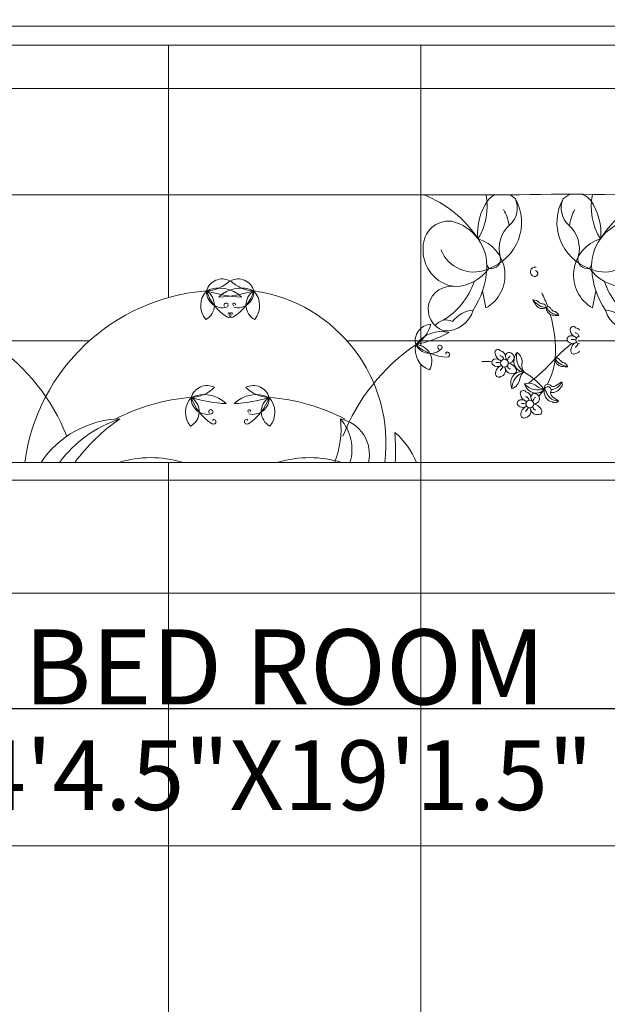
# Model space of a CAD drawing. Units: inches. Extents: x 351 to 1738, y -265 to 286.
# Tile 34 of 38: x 1448 to 1506, y 20 to 118. Entities that reach past the tile are written whole.
import ezdxf

# ---------------------------------------------------------------- set-up
doc = ezdxf.new("R2010")
doc.units = ezdxf.units.IN
doc.header["$MEASUREMENT"] = 0
for name, color, linetype, lineweight in [('A-ANNO-DIMS', 2, 'Continuous', 18), ('A-AREA-IDEN', 7, 'Continuous', 18), ('A-FLOR-PATT', 9, 'Continuous', 9), ('A-FURN', 18, 'Continuous', 13)]:
    doc.layers.add(name, color=color, linetype=linetype, lineweight=lineweight)
doc.styles.add('Annotative', font='arial.ttf')
doc.styles.get("Standard").update_dxf_attribs({"font": 'arial.ttf'})
doc.dimstyles.get("Standard").update_dxf_attribs({"dimtxt": 8, "dimasz": 5, "dimexe": 0.18, "dimexo": 0.0625, "dimgap": 0.09, "dimtad": 1, "dimtoh": 1, "dimzin": 0, "dimdsep": 46, "dimlunit": 4, "dimtxsty": 'Standard', "dimcen": 0, "dimclre": 256, "dimadec": 0, "dimazin": 0, "dimtfac": 1, "dimtofl": 0, "dimtmove": 0, "dimatfit": 3, "dimfxl": 1, "dimtolj": 1, "dimtzin": 0, "dimlwe": -1, "dimarcsym": 0})

# ---------------------------------------------------------------- blocks, each defined once
blk = doc.blocks.new('BED-DOUBLE-W-NIGHTSTANDS')
for p, q in [((121.406, 44.947), (28.441, 44.947)), ((121.549, 43.065), (28.441, 43.065)), ((106.084, 28.242), (44.816, 28.242)), ((102.765, 17.047), (102.431, 18.753)), ((113.311, 17.047), (113.645, 18.753))]:
    blk.add_line(p, q)
for points in [[(121.562, 54.359), (129.93, 54.359), (129.93, 0), (19.917, 0), (19.917, 54.359), (28.453, 54.359)], [(28.449, 52.61), (21.666, 52.61), (21.666, 1.749), (128.181, 1.749), (128.181, 52.61), (121.53, 52.61)]]:
    blk.add_lwpolyline(points)
for centre in [(104.593, 11.579), (107.107, 7.529)]:
    blk.add_circle(centre, 0.384)
for centre, radius, start, end in [((110.705, -118.523), 146.838, 85.24024, 91.80351), ((111.698, 26.573), 1.817, 106.63434, 135.54831), ((111.698, 26.573), 1.817, 37.67503, 72.58143), ((119.442, 27.126), 6.252, 169.24899, 211.17822), ((92.445, 17.616), 11.421, 33.66712, 68.50587), ((107.751, 24.412), 5.82, 145.78505, 184.73037), ((96.634, 27.126), 6.252, 328.82178, 10.28665), ((104.377, 26.573), 1.817, 113.28564, 142.32497), ((101.476, 25.502), 4.809, 289.28218, 29.1751), ((104.377, 26.573), 1.817, 44.45169, 66.71436), ((103.609, 26.933), 2.258, 311.56531, 23.83541), ((114.6, 25.502), 4.809, 150.8249, 250.71782), ((112.466, 26.933), 2.258, 156.16459, 228.43469), ((108.324, 24.412), 5.82, 355.26963, 34.21495), ((123.631, 17.616), 11.421, 113.64533, 146.33288), ((100.75, 24.631), 4.338, 7.43599, 29.91487), ((115.326, 24.631), 4.338, 150.08513, 172.56401), ((99.098, 23.1), 2.548, 84.48557, 181.05378), ((98.316, 21.215), 4.539, 355.29334, 76.921), ((117.76, 21.215), 4.539, 103.079, 184.70666), ((107.16, 22.929), 3.094, 131.56531, 195.14713), ((108.916, 22.929), 3.094, 344.85287, 48.43469), ((100.894, 20.299), 3.752, 299.90854, 73.1337), ((115.181, 20.299), 3.752, 106.8663, 240.09146), ((100.143, 22.735), 3.606, 174.94485, 262.88575), ((101.56, 24.102), 3.502, 201.58187, 291.42215), ((114.516, 24.102), 3.502, 248.57785, 338.41813), ((103.27, 21.876), 0.937, 257.30406, 15.14713), ((112.806, 21.876), 0.937, 164.85287, 282.69594), ((99.516, 23.537), 4.383, 272.3591, 324.04014), ((94.756, 21.336), 8.098, 326.28828, 356.5076), ((107.751, 24.412), 5.82, 212.70113, 216.34448), ((107.638, 20.635), 0.473, 79.58644, 259.56155), ((107.605, 20.456), 0.291, 259.56155, 77.29493), ((108.324, 24.412), 5.82, 323.65552, 327.29887), ((116.56, 23.537), 4.383, 215.95986, 267.6409), ((121.319, 21.336), 8.098, 183.4924, 213.71172), ((76.659, 18.283), 1.634, 63.02737, 163.80375), ((75.004, 22.103), 3.366, 271.45846, 315.37266), ((78.218, 18.283), 1.634, 16.19625, 116.97263), ((79.873, 22.103), 3.366, 224.62734, 268.54154), ((94.823, 21.91), 7.124, 301.26137, 341.7045), ((121.253, 21.91), 7.124, 198.2955, 238.73863), ((76.623, -0.907), 19.706, 94.46233, 172.25504), ((76.708, 17.271), 2.185, 137.78732, 219.11446), ((74.227, 17.338), 1.646, 298.5391, 58.36268), ((76.701, 18.676), 1.612, 177.75849, 283.85198), ((76.373, 15.9), 3.115, 45.54113, 114.31008), ((79.214, 31.893), 13.785, 252.59304, 267.25817), ((79.804, 20.354), 4.984, 198.91595, 238.01098), ((78.505, 15.9), 3.115, 65.68992, 134.45887), ((75.663, 31.893), 13.785, 272.74183, 287.40696), ((75.073, 20.354), 4.984, 301.98902, 341.08405), ((78.176, 18.676), 1.612, 256.14802, 2.24151), ((80.65, 17.338), 1.646, 121.63732, 241.4609), ((78.169, 17.271), 2.185, 320.88554, 42.21268), ((77.617, 3.643), 15.251, 352.86355, 81.81966), ((99.313, 16.925), 2.265, 80.26398, 250.86884), ((97.145, 12.86), 12.498, 20.10592, 26.9968), ((107.447, 17.052), 0.792, 39.50559, 92.64212), ((109.278, 19.327), 2.385, 218.43876, 238.83597), ((111.218, 19.743), 4.256, 206.50636, 215.31021), ((109.029, 19.778), 2.424, 246.39009, 254.48709), ((77.036, 17.318), 0.213, 283.85198, 219.92454), ((77.821, 17.4), 0.128, 320.19092, 256.02088), ((98.77, 17.606), 2.828, 265.96902, 344.3045), ((101.816, 13.847), 3.012, 96.1662, 141.58255), ((108.328, 17.714), 0.724, 216.52319, 302.46683), ((108.698, 18.368), 1.265, 238.83597, 270.81412), ((108.411, 17.136), 0.307, 353.94573, 95.62162), ((109.439, 17.049), 0.724, 175.71315, 261.65678), ((108.889, 16.849), 0.307, 22.55835, 124.23425), ((109.84, 17.685), 1.265, 207.36586, 239.34401), ((110.926, 18.642), 2.424, 223.69288, 231.78988), ((110.411, 18.648), 2.385, 239.34401, 259.74122), ((109.271, 15.96), 0.792, 25.53786, 78.67439), ((117.306, 17.606), 2.828, 195.6955, 274.03098), ((114.26, 13.847), 3.012, 38.41745, 83.8338), ((77.294, 16.335), 0.245, 238.01098, 71.55918), ((77.334, 16.455), 0.119, 71.55918, 188.01668), ((77.583, 16.335), 0.245, 108.44082, 301.98902), ((77.543, 16.455), 0.119, 351.98332, 108.44082), ((98.847, 14.471), 1.388, 63.97555, 143.26805), ((97.145, 12.86), 12.498, 356.17232, 16.41582), ((109.862, 20.555), 4.256, 262.86976, 271.67361), ((97.395, 13.794), 1.634, 92.95159, 193.72796), ((94.055, 16.28), 3.366, 301.38267, 345.29688), ((98.336, 11.586), 3.115, 75.46535, 144.23429), ((111.397, 14.916), 0.297, 35.0752, 194.76444), ((112.026, 14.961), 0.924, 187.49685, 251.27373), ((111.511, 14.458), 0.641, 37.3642, 78.43627), ((92.82, 26.864), 13.785, 282.51726, 297.18239), ((111.128, 13.945), 0.331, 99.6513, 222.32085), ((111.348, 14.146), 0.629, 222.32085, 310.21108), ((111.205, 13.489), 0.794, 46.34618, 99.6513), ((111.356, 12.663), 1.258, 74.28291, 96.91484), ((111.595, 14.227), 0.367, 358.13253, 88.89195), ((112.043, 13.863), 0.384, 93.27684, 266.72316), ((42.91, -2.855), 19.706, 21.40921, 55.61345), ((106.937, -2.855), 19.706, 124.38655, 158.59079), ((97.943, 12.942), 2.185, 167.71153, 249.03868), ((97.235, 14.156), 1.612, 207.6827, 313.77619), ((99.088, 17.159), 4.984, 228.84017, 267.9352), ((95.759, 11.762), 1.646, 328.46331, 88.28689), ((98.203, 13.146), 0.213, 313.77619, 249.71835), ((103.947, 12.632), 0.297, 35.0752, 194.76444), ((104.062, 12.175), 0.641, 3.63497, 78.43627), ((120.068, 2.226), 14.328, 127.9541, 136.84587), ((112.056, 12.814), 0.893, 111.63824, 184.94696), ((111.46, 12.763), 0.295, 184.94696, 307.52629), ((110.834, 13.997), 1.167, 312.38963, 336.57243), ((111.519, 13.152), 0.634, 280.95974, 322.23791), ((98.892, 12.546), 0.119, 101.4834, 217.94089), ((98.917, 12.423), 0.245, 267.9352, 101.4834), ((102.727, 4.223), 7.516, 85.24147, 92.89291), ((103.678, 11.661), 0.331, 99.6513, 222.32085), ((103.755, 11.205), 0.794, 46.34618, 99.6513), ((104.576, 12.677), 0.924, 187.49685, 251.27373), ((104.145, 11.943), 0.367, 358.13253, 88.89195), ((105.076, 12.256), 0.377, 48.29465, 186.24744), ((105.304, 12.26), 0.604, 184.21229, 228.15875), ((105.43, 11.809), 0.529, 118.84925, 179.93549), ((105.017, 12.114), 0.524, 268.57189, 53.89544), ((106.805, 11.798), 1.273, 138.34199, 184.98936), ((107.535, 12.15), 1.752, 163.63009, 235.46314), ((105.103, 11.659), 1.239, 352.07481, 52.68955), ((94.351, 25.887), 20.619, 307.82556, 317.75876), ((103.371, 12.545), 6.266, 330.79592, 355.24398), ((110.338, 11.972), 0.724, 175.71315, 261.65678), ((109.788, 11.772), 0.307, 22.55835, 124.23425), ((110.739, 12.607), 1.265, 207.36586, 239.34401), ((111.825, 13.564), 2.424, 223.69288, 231.78988), ((103.898, 11.862), 0.629, 222.32085, 310.21108), ((104.606, 10.53), 0.893, 111.63824, 184.94696), ((103.906, 10.379), 1.258, 74.28291, 96.91484), ((103.384, 11.713), 1.167, 312.38963, 336.57243), ((104.069, 10.868), 0.634, 280.95974, 28.78041), ((105.375, 11.286), 0.758, 188.56141, 292.59143), ((105.162, 11.255), 0.255, 172.86802, 277.09399), ((104.696, 10.418), 1.212, 31.9501, 75.24419), ((106.296, 9.683), 1.065, 91.4625, 159.4747), ((106.599, 11.759), 1.065, 183.87739, 267.15012), ((105.401, 10.858), 0.381, 314.37319, 31.9501), ((102.727, 4.223), 7.516, 66.15226, 66.94993), ((107.351, 11.346), 1.031, 172.07481, 218.23927), ((111.31, 13.571), 2.385, 239.34401, 259.74122), ((110.761, 15.478), 4.256, 262.86976, 271.67361), ((110.17, 10.882), 0.792, 25.53786, 78.67439), ((104.01, 10.479), 0.295, 184.94696, 307.52629), ((106.482, 9.587), 1.273, 158.36273, 205.0101), ((107.08, 9.04), 1.752, 107.88895, 179.722), ((104.891, 10.208), 1.239, 290.66254, 351.27729), ((107.135, 9.864), 1.031, 125.11283, 171.27729), ((102.727, 4.223), 7.516, 40.18202, 59.45598), ((75.15, 7.729), 1.634, 63.02737, 163.80375), ((73.496, 11.549), 3.366, 271.45846, 315.37266), ((79.727, 7.729), 1.634, 16.19625, 116.97263), ((81.381, 11.549), 3.366, 224.62734, 268.54154), ((106.461, 8.581), 0.297, 35.0752, 194.76444), ((107.007, 8.361), 1.239, 49.38119, 109.99593), ((107.907, 10.674), 1.752, 220.93647, 292.76952), ((107.809, 9.869), 1.273, 195.64837, 242.29574), ((107.731, 9.675), 1.065, 241.18377, 321.67918), ((108.485, 10.084), 1.031, 229.38119, 275.54564), ((103.371, 12.545), 6.266, 317.50829, 325.99666), ((109.522, 8.719), 1, 162.8042, 259.69432), ((108.881, 9.155), 0.335, 45.73542, 228.12966), ((108.882, 8.904), 0.335, 338.24522, 160.63946), ((102.58, 6.101), 6.693, 21.70871, 26.21806), ((109.425, 9.714), 0.444, 225.73542, 301.11559), ((109.606, 8.615), 0.444, 158.24522, 233.62539), ((109.296, 9.675), 1, 262.60083, 327.18452), ((109.167, 10.115), 1.162, 272.31716, 340.52013), ((103.853, 18.945), 11.227, 301.11559, 304.8118), ((109.903, 9.493), 0.429, 303.09787, 33.13641), ((75.114, -11.462), 19.706, 94.46233, 117.4146), ((75.2, 6.716), 2.185, 137.78732, 219.11446), ((72.718, 6.783), 1.646, 298.5391, 58.36268), ((75.192, 8.121), 1.612, 177.75849, 283.85198), ((74.864, 5.345), 3.115, 45.54113, 114.31008), ((78.296, 9.8), 4.984, 198.91595, 238.01098), ((77.705, 21.338), 13.785, 252.59304, 267.25817), ((80.013, 5.345), 3.115, 65.68992, 134.45887), ((77.172, 21.338), 13.785, 272.74183, 287.40696), ((76.581, 9.8), 4.984, 301.98902, 341.08405), ((79.685, 8.121), 1.612, 256.14802, 2.24151), ((82.159, 6.783), 1.646, 121.63732, 241.4609), ((79.677, 6.716), 2.185, 320.88554, 42.21268), ((79.763, -11.462), 19.706, 62.5854, 85.53767), ((106.191, 7.611), 0.331, 99.6513, 222.32085), ((106.269, 7.154), 0.794, 46.34618, 99.6513), ((107.09, 8.626), 0.924, 187.49685, 251.27373), ((106.659, 7.892), 0.367, 358.13253, 88.89195), ((106.575, 8.124), 0.641, 3.63497, 78.43627), ((107.589, 8.205), 0.377, 48.29465, 186.24744), ((107.818, 8.209), 0.604, 184.21229, 228.15875), ((107.943, 7.758), 0.529, 118.84925, 179.93549), ((107.531, 8.063), 0.524, 268.57189, 53.89544), ((109.878, 9.007), 1.162, 201.70871, 273.02993), ((116.001, 17.297), 11.227, 233.62539, 237.3216), ((109.585, 8.089), 0.429, 235.60767, 325.6462), ((75.527, 6.763), 0.213, 283.85198, 219.92454), ((79.33, 6.845), 0.128, 320.19092, 256.02088), ((106.411, 7.811), 0.629, 222.32085, 310.21108), ((107.12, 6.48), 0.893, 111.63824, 184.94696), ((106.42, 6.328), 1.258, 74.28291, 96.91484), ((105.898, 7.662), 1.167, 312.38963, 336.57243), ((106.583, 6.817), 0.634, 280.95974, 28.78041), ((107.889, 7.235), 0.758, 188.56141, 292.59143), ((107.676, 7.205), 0.255, 172.86802, 277.09399), ((107.209, 6.368), 1.212, 31.9501, 75.24419), ((107.914, 6.807), 0.381, 314.37319, 31.9501), ((66.738, -3.546), 9.602, 91.27197, 146.53828), ((70.192, -5.336), 11.966, 107.85038, 143.69643), ((76.481, -8.7), 17.799, 124.01234, 144.05304), ((75.785, 5.781), 0.245, 238.01098, 71.55918), ((75.825, 5.9), 0.119, 71.55918, 188.01668), ((79.092, 5.781), 0.245, 108.44082, 301.98902), ((79.052, 5.9), 0.119, 351.98332, 108.44082), ((79.589, 5.037), 8.823, 338.11703, 6.61954), ((87.682, 2.581), 3.537, 346.38982, 79.07385), ((85.024, 3.067), 4.473, 342.86088, 41.90487), ((106.524, 6.428), 0.295, 184.94696, 307.52629), ((66.54, 2.982), 27.264, 357.40811, 3.65191), ((88.487, -1.325), 8.012, 22.55474, 48.95456), ((69.603, -8.612), 10.836, 73.54311, 107.0202), ((85.274, -8.612), 10.836, 72.9798, 106.45689), ((73.896, -14.197), 16.023, 94.37872, 95.63574), ((82.335, -25.174), 28.633, 109.72171, 109.90284), ((80.981, -14.197), 16.023, 84.36426, 85.62128), ((72.542, -25.174), 28.633, 70.09716, 70.27829)]:
    blk.add_arc(centre, radius, start, end)
blk = doc.blocks.new('*D46')
at = {"layer": 'A-ANNO-DIMS', "transparency": 16777216}
for p, q in [((1391.393, 72.125), (1391.393, 49.373)), ((1542.294, 72.125), (1542.294, 49.373))]:
    blk.add_line(p, q, dxfattribs=at)
at = {"layer": 'A-ANNO-DIMS', "color": 0, "lineweight": -2, "transparency": 16777216}
for p, q in [((1396.393, 49.553), (1537.294, 49.553)), ((1542.294, 49.553), (1738.088, 49.553))]:
    blk.add_line(p, q, dxfattribs=at)
at = {"layer": 'A-ANNO-DIMS', "color": 0, "transparency": 16777216}
for points in [[(1396.393, 50.386), (1396.393, 48.72), (1391.393, 49.553)], [(1537.294, 50.386), (1537.294, 48.72), (1542.294, 49.553)]]:
    blk.add_solid(points, dxfattribs=at)
at = {"layer": 'Defpoints', "color": 0, "transparency": 16777216}
for p in [(1391.393, 72.188), (1542.294, 72.188), (1542.294, 49.553)]:
    blk.add_point(p, dxfattribs=at)
at = {"layer": 'A-ANNO-DIMS', "color": 0, "transparency": 16777216, "insert": (1642.691, 53.779), "char_height": 8, "attachment_point": 5}
blk.add_mtext('\\A1;BED AND NIGHTSTANDS 12\'-7" TYP.', dxfattribs=at)

msp = doc.modelspace()

# ---------------------------------------------------------------- hatches: boundary and pattern name
at = {"layer": 'A-FLOR-PATT', "transparency": 33554559}
h = msp.add_hatch(dxfattribs=at)
h.set_pattern_fill('ANSI37', color=256, scale=200, angle=135)
h.set_pattern_definition([(180, (1112.704, -164.037), (-2e-15, -25), []), (270, (1112.704, -164.037), (25, -5e-15), [])])
h.paths.add_polyline_path([(1380.064, 73.463), (1380.132, 148.463), (1338.064, 148.463), (1290.704, 148.463), (1290.704, 88.463), (1248.704, 88.463), (1248.704, -2.009), (1244.704, -2.009), (1244.704, 142.457), (1160.704, 142.457), (1160.704, 158.963), (1160.704, 170.137), (1160.704, 206.137), (1160.704, 228.963), (1112.704, 228.963), (1112.704, 209.963), (1112.704, 168.963), (1124.704, 168.963), (1124.704, 162.963), (1112.704, 162.963), (1112.704, 64.463), (1112.704, 60.463), (1112.704, 0.463), (1112.704, -48.026), (1146.804, -47.981), (1146.804, -35.691), (1207.804, -35.691), (1207.804, -47.902), (1236.542, -47.864), (1236.544, -50.009), (1248.5, -50.009), (1248.506, -102.915), (1248.512, -150.915), (1248.514, -164.037), (1248.549, -164.037), (1273.017, -164.037), (1273.017, -128.799), (1355.24, -128.799), (1355.24, -164.037), (1384.204, -164.037), (1384.204, -57.037), (1380.064, -57.037), (1380.064, -48.037), (1392.064, -48.037), (1392.064, -53.037), (1406.549, -53.037), (1406.549, -57.037), (1401.204, -57.037), (1401.204, -147.037), (1468.204, -147.037), (1468.204, -138.5), (1472.204, -138.5), (1472.204, -102.5), (1468.204, -102.5), (1468.204, -57.037), (1442.549, -57.037), (1442.549, -53.037), (1463.049, -53.037), (1463.049, -40.747), (1524.049, -40.747), (1524.049, -48.037), (1536.064, -48.037), (1536.064, -53.037), (1557.704, -53.037), (1557.704, 204.963), (1384.204, 204.963), (1384.204, 73.463), (1392.064, 73.463), (1392.064, 64.463), (1384.204, 64.463), (1384.204, -3.5), (1380.204, -3.537), (1380.204, 64.463), (1380.064, 64.463)])
h.paths.add_polyline_path([(1510.714, 86.458, -0.103984), (1511.661, 85.595, 0.470438), (1510.158, 87.614, 0.0961)], flags=16)
h.paths.add_polyline_path([(1510.443, 100.266, 0.009798), (1504.693, 100.48, 0.02879), (1504.6, 99.767, -0.165331), (1505.519, 96.135, -0.143601)], flags=16)
h.paths.add_polyline_path([(1487.201, 85.595, -0.103984), (1488.148, 86.458, 0.0961), (1488.704, 87.614, 0.470438)], flags=0)
h.paths.add_polyline_path([(1495.052, 100.43), (1494.178, 100.43, -0.026463), (1494.262, 99.774, -0.144219)], flags=16)
h.paths.add_polyline_path([(1444.485, 86.458, -0.103984), (1445.433, 85.595, 0.470438), (1443.93, 87.614, 0.0961)], flags=16)
h.paths.add_polyline_path([(1420.972, 85.595, -0.103984), (1421.92, 86.458, 0.0961), (1422.475, 87.614, 0.470438)], flags=16)
h.paths.add_polyline_path([(1428.632, 100.335, 0.001054), (1427.971, 100.309, -0.021524), (1428.033, 99.774, -0.114301)], flags=16)
h.paths.add_polyline_path([(1419.906, 143.708, 0.024979), (1420.222, 157.526), (1421.573, 159.101), (1421.573, 175.369), (1391.393, 175.369), (1391.393, 200.519), (1542.294, 200.519), (1542.294, 175.369), (1512.028, 175.369, 0.019865), (1511.521, 153.838, 0.025134), (1512.758, 118.323, 0.020553), (1512.942, 115.253), (1419.834, 115.253, -0.000414), (1419.843, 124.798), (1413.059, 124.798), (1413.059, 84.437, -0.061853), (1415.831, 80.45, -0.093077), (1420.972, 85.595, -0.267537), (1422.371, 84.732, 0.08511), (1424.052, 84.616, -0.885393), (1424.033, 84.851, -1.125815), (1424.073, 84.366, -0.087987), (1422.371, 84.732, -0.267537), (1422.326, 83.089, -0.370542), (1420.972, 85.595, 0.093077), (1415.831, 80.45, -0.087414), (1417.914, 73.937), (1418.941, 73.937, 0.02725), (1418.913, 76.906, -0.115703), (1421.051, 73.937), (1445.354, 73.937, -0.115703), (1447.492, 76.906, 0.02725), (1447.464, 73.937), (1448.491, 73.937, -0.087414), (1450.574, 80.45, 0.093077), (1445.433, 85.595, -0.370542), (1444.079, 83.089, -0.267537), (1444.034, 84.732, -0.087987), (1442.332, 84.366, -1.125815), (1442.372, 84.851, -2.032736), (1442.364, 84.368, 0.086378), (1444.034, 84.732, -0.267537), (1445.433, 85.595, -0.093077), (1450.574, 80.45, -0.257732), (1466.483, 90.927, -0.47867), (1468.832, 91.907, -0.47867), (1471.18, 90.927, -0.26264), (1483.053, 81.78, -0.071866), (1487.201, 85.595, -0.267537), (1488.6, 84.732, 0.08511), (1490.28, 84.616, -0.885393), (1490.262, 84.851, -1.125815), (1490.301, 84.366, -0.087987), (1488.6, 84.732, -0.267537), (1488.554, 83.089, -0.370542), (1487.201, 85.595, 0.071866), (1483.053, 81.78, -0.132065), (1484.143, 73.937), (1485.169, 73.937, 0.02725), (1485.142, 76.906, -0.115703), (1487.28, 73.937), (1511.582, 73.937, -0.115703), (1513.72, 76.906, 0.02725), (1513.693, 73.937), (1514.719, 73.937, -0.087414), (1516.802, 80.45, 0.093077), (1511.661, 85.595, -0.370542), (1510.308, 83.089, -0.267537), (1510.262, 84.732, -0.087987), (1508.561, 84.366, -1.125815), (1508.601, 84.851, -2.032736), (1508.592, 84.368, 0.086378), (1510.262, 84.732, -0.267537), (1511.661, 85.595, -0.093077), (1516.802, 80.45, -0.061853), (1519.575, 84.437), (1519.575, 73.937), (1413.059, 73.937), (1413.059, 124.798), (1419.843, 124.798, -0.000821)], flags=16)
h.paths.add_polyline_path([(1220.149, 54.133, -0.103984), (1220.869, 53.476, 0.470438), (1219.727, 55.011, 0.0961)], flags=16)
h.paths.add_polyline_path([(1219.944, 64.626, 0.009798), (1215.574, 64.789, 0.02879), (1215.503, 64.247, -0.165331), (1216.201, 61.487, -0.143601)], flags=16)
h.paths.add_polyline_path([(1209.779, 64.449, 0.097446), (1209.339, 64.751), (1208.247, 64.751, 0.12739), (1207.7, 64.326, 0.171586), (1206.95, 61.475, -0.158854), (1207.636, 59.45, 0.015898), (1207.795, 59.218, 0.061546), (1208.598, 59.616, 0.175416), (1208.638, 60.099, -0.284779), (1209.348, 62.472, 0.326216)], flags=16)
h.paths.add_polyline_path([(1169.818, 54.133, -0.103984), (1170.538, 53.476, 0.470438), (1169.396, 55.011, 0.0961)], flags=16)
h.paths.add_polyline_path([(1159.017, 62.472, 0.284764), (1158.307, 60.099, -0.175433), (1158.267, 59.616, 0.39293), (1159.448, 64.449, -0.32623)], flags=16)
h.paths.add_polyline_path([(1156.342, 58.239, -0.178321), (1154.011, 55.31, -0.174736), (1154.722, 55.233, -0.200802), (1156.27, 56.086, 0.12699), (1157.283, 58.991, -0.091205)], flags=16)
h.paths.add_polyline_path([(1156.624, 61.413, 0.157275), (1157.316, 64.247, 0.169622)], flags=16)
h.paths.add_polyline_path([(1152.67, 54.133, -0.0961), (1151.95, 53.476, 0.064076), (1154.465, 54.384, 0.199016)], flags=16)
h.paths.add_polyline_path([(1202.281, 53.476, -0.103984), (1203, 54.133, 0.0961), (1203.423, 55.011, 0.470438)], flags=0)
h.paths.add_polyline_path([(1151.139, 97.64, 0.024979), (1151.379, 108.141), (1152.406, 109.338), (1152.406, 121.701), (1129.47, 121.701), (1129.47, 140.814), (1244.149, 140.814), (1244.149, 121.701), (1221.148, 121.701, 0.019865), (1220.763, 105.338, 0.025134), (1221.703, 78.349, 0.020553), (1221.843, 76.016), (1151.078, 76.016, -0.128743), (1148.786, 65.037, 0.539352), (1150.327, 64.171, -0.027594), (1163.481, 64.751, 0.097695), (1163.04, 64.449, 0.326216), (1163.471, 62.472, -0.284777), (1164.181, 60.099, -0.194757), (1165.846, 61.443, -0.155402), (1165.172, 64.247, -0.166022), (1165.869, 61.475, -0.177014), (1167.852, 62.77, -0.448203), (1169.974, 60.807, -0.393499), (1167.679, 57.86, -0.895548), (1168.438, 54.524, -0.355767), (1166.218, 56.086, -0.066024), (1165.505, 57.539), (1165.251, 56.243, -0.371732), (1164.02, 59.758, -0.373614), (1163.04, 64.449, -0.097695), (1163.481, 64.751, 0.021354), (1153.294, 64.429, -0.134183), (1156.695, 61.368, 0.186873), (1154.636, 62.77, 0.448203), (1152.514, 60.807, 0.403726), (1154.905, 57.846, 0.711219), (1153.334, 55, 0.53154), (1151.95, 53.476, -0.267537), (1153.013, 52.821, 0.08511), (1154.29, 52.732, -0.885393), (1154.276, 52.911, -1.125815), (1154.306, 52.543, -0.087987), (1153.013, 52.821, -0.267537), (1152.978, 51.572, -0.370542), (1151.95, 53.476, 0.093077), (1148.043, 49.566, -0.087414), (1149.626, 44.617), (1150.406, 44.617, 0.02725), (1150.385, 46.873, -0.115703), (1152.01, 44.617), (1170.478, 44.617, -0.115703), (1172.103, 46.873, 0.02725), (1172.082, 44.617), (1172.862, 44.617, -0.087414), (1174.445, 49.566, 0.093077), (1170.538, 53.476, -0.370542), (1169.51, 51.572, -0.267537), (1169.475, 52.821, -0.087987), (1168.182, 52.543, -1.125815), (1168.212, 52.911, -2.032736), (1168.206, 52.544, 0.086378), (1169.475, 52.821, -0.267537), (1170.538, 53.476, -0.093077), (1174.445, 49.566, -0.257732), (1186.536, 57.528, -0.47867), (1188.321, 58.273, -0.47867), (1190.106, 57.528, -0.26264), (1199.128, 50.577, -0.071866), (1202.281, 53.476, -0.267537), (1203.344, 52.821, 0.08511), (1204.621, 52.732, -0.885393), (1204.607, 52.911, -1.125815), (1204.637, 52.543, -0.087987), (1203.344, 52.821, -0.267537), (1203.309, 51.572, -0.370542), (1202.281, 53.476, 0.071866), (1199.128, 50.577, -0.132065), (1199.957, 44.617), (1200.737, 44.617, 0.02725), (1200.716, 46.873, -0.115703), (1202.341, 44.617), (1220.809, 44.617, -0.115703), (1222.434, 46.873, 0.02725), (1222.413, 44.617), (1223.193, 44.617, -0.087414), (1224.776, 49.566, 0.093077), (1220.869, 53.476, -0.370542), (1219.841, 51.572, -0.267537), (1219.806, 52.821, -0.087987), (1218.513, 52.543, -1.125815), (1218.543, 52.911, -2.032736), (1218.537, 52.544, 0.086378), (1219.806, 52.821, -0.267537), (1220.869, 53.476, -0.093077), (1224.776, 49.566, -0.061853), (1226.883, 52.597), (1226.883, 44.617), (1145.936, 44.617), (1145.936, 83.269), (1151.091, 83.269, -0.000821)], flags=16)
h.paths.add_polyline_path([(1218.01, 57.86, -0.895548), (1218.769, 54.524, -0.355767), (1216.549, 56.086, -0.066024), (1215.836, 57.539), (1215.582, 56.243, -0.371732), (1214.351, 59.758, -0.373614), (1213.371, 64.449, 0.326216), (1213.802, 62.472, -0.284777), (1214.512, 60.099, -0.194757), (1216.177, 61.443, -0.179991), (1218.183, 62.77, -0.448203), (1220.305, 60.807, -0.393499)], flags=16)
h.paths.add_polyline_path([(1424.735, 91.363, -0.393499), (1421.715, 95.241, -0.448203), (1424.507, 97.824, -0.179991), (1427.147, 96.077, -0.194757), (1429.338, 94.309, -0.284777), (1430.272, 97.432, 0.326216), (1430.839, 100.034, -0.373614), (1429.55, 93.861, -0.371732), (1427.929, 89.235), (1427.596, 90.941, -0.066024), (1426.657, 89.029, -0.355767), (1423.736, 86.973, -0.895548)], flags=16)
h.paths.add_polyline_path([(1238.033, 131.257, -1), (1227.329, 131.257, -1)], flags=0)
h.paths.add_polyline_path([(1235.357, 131.257, -1), (1230.005, 131.257, -1)], flags=0)
h.paths.add_polyline_path([(1214.039, 54.243, 0.154382), (1214.38, 53.992, 0.358955), (1213.613, 54.016, 0.603948), (1214.379, 53.657, 0.371319), (1213.968, 52.872, 0.187994), (1214.312, 52.809, -0.592455), (1213.953, 52.967, -0.294279), (1214.083, 53.691, -1.300187), (1213.881, 54.134, -0.283762), (1214.469, 53.896, 1.15094)], flags=16)
h.paths.add_polyline_path([(1212.091, 56.286, -0.408434), (1211.337, 56.445, -0.036259), (1211.098, 56.848, -0.236098), (1211.59, 56.63, 0.035345), (1211.835, 56.543, -0.475241), (1212.091, 56.286, -0.475241), (1212.438, 56.182, 0.035345), (1212.631, 56.007, -0.236098), (1213.056, 55.676, -0.036259), (1212.588, 55.697, -0.408434)], flags=16)
h.paths.add_polyline_path([(1211.469, 50.297, 0.296043), (1210.47, 50.527, 0.310883), (1211.931, 50.148, 0.021255)], flags=16)
h.paths.add_polyline_path([(1213.739, 51.818, -0.036259), (1213.271, 51.838, -0.408434), (1212.774, 52.427, -0.094786), (1212.293, 50.703, 1.150474), (1212.911, 50.232, 0.166288), (1213.265, 50.68, -0.025254), (1212.603, 50.13, 1.087932), (1212.471, 49.407, 0.166288), (1213.02, 49.251, -0.016128), (1212.567, 49.563, -0.286859), (1212.217, 49.638, 0.022156), (1212.046, 50.055, -0.64613), (1212.185, 50.498, 0.088412), (1212.732, 52.077, -1.186037), (1213.121, 52.323, 0.035345), (1213.314, 52.148, -0.236098)], flags=16)
h.paths.add_polyline_path([(1212.094, 50.342, -0.048524), (1211.54, 49.605, -1.103834), (1211.397, 48.738, -0.785515), (1211.683, 48.254, -0.392043), (1210.948, 48.525, -0.392819), (1210.561, 47.995, -0.592455), (1210.201, 48.153, -0.294279), (1210.331, 48.877, -0.704172), (1210.316, 49.592, -0.679344), (1210.729, 50.112, 0.563676)], flags=16)
h.paths.add_polyline_path([(1211.274, 49.829, -0.139826), (1210.745, 49.859, -0.217879), (1210.948, 49.509, -0.498572)], flags=0)
h.paths.add_polyline_path([(1433.426, 81.49, -0.181571), (1434.245, 81.788, -0.008067), (1433.726, 82.205, 0.045578), (1432.755, 81.242, 0.179011)], flags=16)
h.paths.add_polyline_path([(1434.146, 81.009, -0.132442), (1433.645, 80.771, 0.259089), (1433.234, 80.471, -0.180211), (1433.392, 80.805, -0.16994), (1432.758, 81.109, 0.032652), (1433.273, 80.474, -0.493363), (1434.046, 80.146, -0.390497)], flags=16)
h.paths.add_polyline_path([(1434.83, 80.047, -0.947538), (1435.294, 79.576, -0.299128), (1434.625, 79.404, -0.270439), (1435.01, 78.591, -0.592455), (1434.537, 78.382, -0.392819), (1434.027, 79.08, -0.392043), (1433.06, 78.723, -0.352042), (1433.003, 79.197, -0.197216), (1433.75, 79.734, -0.71364), (1434.447, 79.939, -0.21479), (1434.819, 80.475, 0.408833), (1435.075, 80.803, -0.226152)], flags=16)
h.paths.add_polyline_path([(1432.67, 81.217, -0.454218), (1431.897, 79.923, -0.414411), (1431.301, 80.035, 0.016129), (1431.897, 80.445, 0.27957), (1432.073, 80.871, -0.289504), (1431.103, 81.321, -0.414411), (1430.978, 81.915, 0.01613), (1431.586, 81.521, 0.341293), (1432.125, 81.583, -0.813186)], flags=16)
h.paths.add_polyline_path([(1429.893, 86.381, -0.947538), (1430.358, 85.91, -0.173106), (1429.984, 85.712, -0.038817), (1431.625, 84.214, -0.0879), (1432.097, 88.549, -0.049768), (1431.254, 88.49, -0.236098), (1431.814, 88.925, 0.035345), (1432.067, 89.155, -0.475241), (1432.524, 89.291, -0.475241), (1432.86, 89.63, 0.035345), (1433.182, 89.744, -0.236098), (1433.83, 90.032, -0.036259), (1433.516, 89.502, -0.408434), (1432.524, 89.291, -0.312424), (1432.106, 88.58, 0.088559), (1431.625, 84.214, -0.408434), (1430.971, 83.439, -0.036259), (1430.355, 83.412, -0.236098), (1430.914, 83.847, 0.035345), (1431.168, 84.078, -0.475241), (1431.625, 84.214, 0.038817), (1429.984, 85.712, -0.321732), (1429.333, 86.048, -0.32743), (1429.883, 86.809, 0.408833), (1430.138, 87.138, -0.226152)], flags=16)
h.paths.add_polyline_path([(1211.206, 58.616, -0.999784), (1211.336, 59.323, -0.614994)], flags=16)
h.paths.add_polyline_path([(1210.288, 49.429, 0.154382), (1210.629, 49.178, 0.358955), (1209.861, 49.202, 0.603948), (1210.627, 48.843, -0.534825), (1210.806, 49.295, 0.748346)], flags=16)
h.paths.add_polyline_path([(1209.589, 51.828, -0.008791), (1209.775, 51.753, 0.112231), (1209.466, 52.019, 1.418851), (1209.014, 51.708, -0.458726), (1208.651, 51.073, -0.592455), (1208.291, 51.232, -0.294279), (1208.421, 51.955, -1.300187), (1208.219, 52.398, -0.226005), (1208.719, 52.257, -0.475519), (1209.158, 52.369, -1.455499), (1209.603, 52.664, 0.421305), (1209.191, 52.262, -0.591212), (1208.979, 51.796, 0.497399), (1209.773, 51.333, 0.649312)], flags=16)
h.paths.add_polyline_path([(1208.029, 52.041, 0.544667), (1208.832, 52.045, 0.220132)], flags=0)
h.paths.add_polyline_path([(1210.438, 51.425, -0.2042), (1210.277, 52.018, 0.270826), (1209.915, 52.897, 0.324115)], flags=0)
h.paths.add_polyline_path([(1209.668, 52.407, -0.60139), (1208.99, 52.221, -0.394916), (1208.248, 52.83, -0.836792), (1208.651, 53.017, -0.338488), (1209.039, 52.571, 0.194138), (1209.191, 52.262, 0.413995), (1209.712, 52.475, 0.51771), (1210.503, 51.416, 0.401922), (1209.493, 50.93, 0.206396), (1209.516, 50.165, -0.319463), (1210.417, 51.418, -0.466635)], flags=16)
h.paths.add_polyline_path([(1206.601, 56.086, -0.355767), (1204.381, 54.524, -0.921198), (1205.236, 57.846, 0.206569), (1207.614, 58.991, -0.12699)], flags=16)
h.paths.add_polyline_path([(1435.487, 82.816, 0.527765), (1436.615, 83.361, 0.50854), (1437.05, 82.433, 0.592455), (1437.524, 82.641, 0.331245), (1436.963, 83.548, 0.387863), (1437.808, 83.626, 0.592954), (1437.618, 84.176, 0.226016), (1436.961, 83.99, 0.318205), (1437.588, 84.854, 0.689374), (1437.05, 84.991, 0.335765), (1436.539, 84.41, -0.156993), (1436.404, 84.065, -0.434611), (1436.961, 83.99, -0.21479), (1437.333, 84.526, 0.408833), (1437.588, 84.854, -0.226152), (1437.343, 84.097, -0.947538), (1437.808, 83.626, -0.299128), (1437.139, 83.455, -0.270439), (1437.524, 82.641, -0.592455), (1437.05, 82.433, -0.392819), (1436.541, 83.13, -0.43966), (1435.475, 82.794, -0.174614), (1435.942, 82.244, -0.206396), (1435.912, 81.237, -0.270826), (1435.125, 82.208, 0.207976), (1434.686, 82.904, -0.196495)], flags=16)
h.paths.add_polyline_path([(1435.386, 84.832, 0.270811), (1434.91, 83.676, -0.204217), (1434.699, 82.895, 0.324115)], flags=0)
h.paths.add_polyline_path([(1435.68, 84.18, -0.217656), (1435.554, 83.304, -0.176705), (1436.236, 83.778, -0.373036)], flags=0)
h.paths.add_polyline_path([(1435.566, 100.034, 0.326216), (1436.133, 97.432, -0.284777), (1437.067, 94.309, -0.194757), (1439.258, 96.077, -0.155402), (1438.371, 99.767, -0.166022), (1439.289, 96.12, -0.177014), (1441.897, 97.824, -0.448203), (1444.69, 95.241, -0.393499), (1441.67, 91.363, -0.895548), (1442.669, 86.973, -0.355767), (1439.748, 89.029, -0.066024), (1438.809, 90.941), (1438.476, 89.235, -0.371732), (1436.855, 93.861, -0.373614)], flags=16)
h.paths.add_polyline_path([(1191.252, 49.507, -0.274022), (1190.658, 48.409, 0.267537), (1191.311, 47.344, 0.370542)], flags=0)
h.paths.add_polyline_path([(1190.301, 49.717, 0.199016), (1188.619, 49.04, 0.064076), (1191.252, 49.507, -0.0961)], flags=0)
h.paths.add_polyline_path([(1189.518, 47.857, 1.125815), (1189.676, 47.523, 2.044605)], flags=0)
h.paths.add_polyline_path([(1464.974, 80.372, 0.274022), (1465.756, 78.927, -0.083013)], flags=0)
h.paths.add_polyline_path([(1464.974, 80.372, 0.370542), (1464.897, 77.525, 0.576324)], flags=0)
h.paths.add_polyline_path([(1464.974, 80.372, -0.470438), (1467.284, 81.372, -0.0961), (1466.226, 80.648, -0.199016), (1468.439, 79.757, -0.064076)], flags=0)
h.paths.add_polyline_path([(1189.511, 56.43, -0.259467), (1188.321, 56.391, -0.259467), (1187.13, 56.43, 0.08511), (1188.193, 55.716, -0.885393), (1188.27, 55.878, -1.196013), (1188.355, 55.442, 0.101459)], flags=0)
h.paths.add_polyline_path([(1188.321, 57.596, 0.078072), (1187.678, 57.24, 0.01555), (1188.321, 57.136, 0.01555), (1188.964, 57.24, 0.078072)], flags=0)
h.paths.add_polyline_path([(1190.164, 55.365, -0.576324), (1190.106, 57.528, -0.198294), (1188.321, 58.319, -0.198294), (1186.536, 57.528, -0.576324), (1186.477, 55.365, -0.370542), (1186.536, 57.528, 0.198294), (1188.321, 58.319, 0.198294), (1190.106, 57.528, -0.370542)], flags=0)
h.paths.add_polyline_path([(1188.372, 55.878, 1.125814), (1188.529, 55.544, 2.044605)], flags=0)
h.paths.add_polyline_path([(1186.341, 49.717, -0.0961), (1185.389, 49.507, 0.064076), (1188.022, 49.04, 0.199016)], flags=0)
h.paths.add_polyline_path([(1185.389, 49.507, -0.267537), (1185.984, 48.409, 0.08511), (1187.046, 47.695, -0.885393), (1187.123, 47.857, -1.125815), (1186.966, 47.523, -0.087987), (1185.984, 48.409, -0.267537), (1185.331, 47.344, -0.370542)], flags=0)
h.paths.add_polyline_path([(1399.441, 187.944, -1), (1413.525, 187.944, -1)], flags=0)
h.paths.add_polyline_path([(1402.962, 187.944, -1), (1410.004, 187.944, -1)], flags=0)
h.paths.add_polyline_path([(1357.663, -72.245), (1377.272, -72.245), (1377.272, -91.854), (1357.663, -91.854)], flags=16)
h.paths.add_polyline_path([(1467.256, 78.201, -1.125815), (1467.049, 77.761, -2.044605)], flags=0)
h.paths.add_polyline_path([(1468.822, 88.714, 0.941125), (1469.106, 88.316, 1.137152), (1468.765, 88.755, 0.890986), (1468.99, 88.245, 0.094828), (1470.398, 89.481, -0.267537), (1471.18, 90.927, -0.028123), (1469.678, 90.547, -0.028774), (1469.948, 90.311, -0.020327), (1468.832, 90.41, -0.020327), (1467.716, 90.311, -0.028774), (1467.986, 90.547, -0.028123), (1466.483, 90.927, -0.267537), (1467.265, 89.481, 0.08511), (1468.663, 88.542, -1.202316)], flags=0)
h.paths.add_polyline_path([(1178.25, 124.523, -0.119929), (1165.65, 124.145, -0.107349), (1159.133, 124.446, -0.102891), (1159.132, 130.465, -0.074897), (1158.993, 137.956, 0.002027), (1167.844, 137.479, -0.07553), (1180.337, 137.666, -0.075861), (1186.502, 137.688, -0.14099), (1186.272, 130.046, -0.095481), (1186.729, 124.748, -0.10603)], flags=0)
h.paths.add_polyline_path([(1469.225, 79.757, -0.199016), (1471.437, 80.648, -0.0961), (1470.379, 81.372, -0.470438), (1472.689, 80.372, -0.370542), (1472.766, 77.525, -0.267537), (1471.907, 78.927, -0.087986), (1470.615, 77.761, -1.125849), (1470.408, 78.201, -2.032736), (1470.642, 77.778, 0.086378), (1471.907, 78.927, -0.267537), (1472.689, 80.372, -0.064076)], flags=0)
h.paths.add_polyline_path([(1430.423, 186.902, -0.074897), (1430.24, 196.758, 0.002027), (1441.887, 196.131, -0.07553), (1458.326, 196.377, -0.075861), (1466.438, 196.406, -0.14099), (1466.136, 186.35, -0.095481), (1466.737, 179.378, -0.10603), (1455.58, 179.082, -0.119929), (1439, 178.585, -0.107349), (1430.425, 178.981, -0.102891)], flags=0)
h.paths.add_polyline_path([(1162.258, 49.939, 0.335765), (1161.87, 49.497, -0.156994), (1161.767, 49.235, -0.434611), (1162.19, 49.178, -0.21479), (1162.473, 49.585, 1.529195)], flags=16)
h.paths.add_polyline_path([(1161.683, 49.021, 0.581518), (1161.268, 49.583, 0.592761)], flags=16)
h.paths.add_polyline_path([(1162.602, 48.058, 0.371319), (1162.192, 48.843, 0.434533), (1162.88, 48.962, 0.185081), (1162.197, 48.926, 1.121837)], flags=16)
h.paths.add_polyline_path([(1161.443, 48.941, -1.307104), (1161.495, 48.571, -0.217752), (1161.136, 48.254, 0.697303), (1161.871, 49.048, 0.121514)], flags=16)
h.paths.add_polyline_path([(1162.531, 49.429, -0.207084), (1162.05, 49.146, -0.99203)], flags=16)
h.paths.add_polyline_path([(1161.304, 49.578, -0.719667), (1161.513, 50.079, -0.130428), (1160.836, 50.168, 0.039593)], flags=0)
h.paths.add_polyline_path([(1162.036, 50.584, -0.008067), (1161.642, 50.9, 0.029367), (1161.35, 50.297, -0.205788)], flags=16)
h.paths.add_polyline_path([(1162.882, 51.392, -0.124733), (1162.763, 51.828, -0.101191), (1162.399, 51.438, -0.153425)], flags=0)
h.paths.add_polyline_path([(1164.235, 51.85, -0.309107), (1164.513, 51.136, -0.627125), (1163.781, 51.603, -0.685909), (1162.777, 51.219, -0.233285), (1163.303, 50.165, -0.270826), (1162.705, 50.903, 0.2042), (1162.381, 51.425, 0.204182), (1162.542, 52.018, -0.270841), (1162.903, 52.897, -0.127261), (1163.219, 52.529, -1.168681), (1163.781, 52.587, -0.329112), (1164.168, 53.017, -0.836792), (1164.571, 52.83, -0.193341), (1164.391, 52.338, -0.947538), (1164.744, 51.981, -0.299128)], flags=16)
h.paths.add_polyline_path([(1163.598, 51.937, -1.262956), (1163.236, 51.831, 0.012575), (1162.971, 51.721, 0.230657), (1163.151, 52.407, -0.164898), (1163.178, 52.661, -0.44932), (1163.628, 52.262, -0.721477), (1164.154, 52.088, -0.849998)], flags=0)
h.paths.add_polyline_path([(1161.613, 58.616, -0.980413), (1161.525, 59.049, -2.908935)], flags=16)
h.paths.add_polyline_path([(1160.252, 49.166, -0.414411), (1159.799, 49.251, 0.016129), (1160.252, 49.563, 0.27957), (1160.386, 49.887, -0.289504), (1159.649, 50.229, -0.414411), (1159.554, 50.68, 0.01613), (1160.015, 50.381, 0.617885), (1160.526, 50.703, -0.094786), (1160.045, 52.427, -0.140444), (1159.682, 52.042, -0.057856), (1159.3, 51.872, 0.544843), (1160.046, 52.419, -0.088122), (1160.404, 55.721, -0.049768), (1159.763, 55.676, -0.236098), (1160.188, 56.007, 0.035345), (1160.381, 56.182, -0.475241), (1160.728, 56.286, -0.475241), (1160.984, 56.543, 0.035345), (1161.229, 56.63, -0.236098), (1161.721, 56.848, -0.036259), (1161.482, 56.445, -0.408434), (1160.728, 56.286, -0.312424), (1160.411, 55.745, 0.088559), (1160.045, 52.427, 0.107081), (1160.634, 50.498, -0.494798), (1160.839, 50.149, -0.454218)], flags=16)
h.paths.add_polyline_path([(1160.666, 49.808, -2.076528), (1160.828, 50.172, 0.019586)], flags=0)
h.paths.add_polyline_path([(1158.439, 53.992, 0.154382), (1158.78, 54.243, 0.748346), (1158.262, 54.109, -0.338225), (1158.492, 53.839, -0.170816), (1159.124, 53.779, 0.495729), (1158.938, 54.134, 0.226016)], flags=16)
h.paths.add_polyline_path([(1160.045, 52.427, 0.038817), (1158.798, 53.565, -0.119818), (1158.574, 53.586, -0.309107), (1158.851, 52.872, -0.187994), (1158.506, 52.809, 0.592455), (1158.866, 52.967, 0.331245), (1158.44, 53.657, 0.201245), (1158.798, 53.565, -0.034023), (1159.901, 52.578, -0.044253), (1159.698, 52.323, -0.475241)], flags=16)
h.paths.add_polyline_path([(1336.926, -95.392), (1336.926, -117.945), (1291.82, -117.945), (1291.82, -95.392)], flags=16)
h.paths.add_polyline_path([(1357.535, -97.244), (1357.726, -96.697, 0.034844)], flags=16)
h.paths.add_polyline_path([(1376.693, -96.478), (1377.301, -96.5, 0.031497), (1375.907, -96.424), (1357.726, -96.424)], flags=16)
h.paths.add_polyline_path([(1379.403, -119.667, 0.026706), (1380.043, -119.439, -0.015299)], flags=16)
h.paths.add_polyline_path([(1357.726, -120.202), (1357.821, -120.202), (1357.821, -120.201)], flags=16)
h.paths.add_polyline_path([(1354.171, -104.592), (1354.469, -98.672, 0.011138)], flags=16)
h.paths.add_polyline_path([(1355.058, -119.136), (1354.578, -118.539, 0.143164)], flags=16)
h.paths.add_polyline_path([(1378.851, -96.821), (1378.85, -96.82), (1378.85, -96.82, -0.04968), (1380.055, -97.191), (1378.85, -96.82, 0.150054), (1375.135, -97.188), (1375.136, -119.44, -0.00997), (1374.747, -116.649), (1357.726, -116.649, 0.169385), (1357.535, -119.382), (1357.535, -119.382), (1357.535, -119.382, 0.034818), (1357.726, -119.928), (1357.726, -119.928), (1357.726, -119.929, -0.034877), (1357.535, -119.382), (1355.507, -119.382), (1355.317, -119.278), (1357.535, -119.382, -0.169394), (1357.726, -116.649, -0.039151), (1374.686, -116.113, -0.002015), (1374.625, -115.546, 0.115322), (1369.915, -115.474, 0.060921), (1369.922, -101.154, 0.115146), (1374.625, -101.079, -0.002016), (1374.686, -100.513, -0.039151), (1357.726, -99.977), (1374.747, -99.977, -0.009963), (1375.135, -97.188), (1375.135, -97.188, -0.150108)], flags=16)
h.paths.add_polyline_path([(1490.963, 91.363, -0.393499), (1487.944, 95.241, -0.448203), (1490.736, 97.824, -0.179991), (1493.376, 96.077, -0.194757), (1495.567, 94.309, -0.284777), (1496.501, 97.432, 0.326216), (1497.068, 100.034, -0.373614), (1495.778, 93.861, -0.371732), (1494.158, 89.235), (1493.824, 90.941, -0.066024), (1492.886, 89.029, -0.355767), (1489.964, 86.973, -0.895548)], flags=16)
h.paths.add_polyline_path([(1354.86, -97.658), (1355.316, -97.348, 0.101911)], flags=16)
h.paths.add_polyline_path([(1497.063, 83.327, 0.176724), (1496.37, 83.785, -0.405139), (1496.016, 83.384, 0.497399), (1497.06, 82.774, 0.649312), (1496.818, 83.426, -0.008791)], flags=16)
h.paths.add_polyline_path([(1496.339, 83.783, 0.592761), (1496.886, 84.522, 0.581518)], flags=16)
h.paths.add_polyline_path([(1495.11, 82.641, 0.592455), (1495.583, 82.433, 0.676915), (1495.805, 83.59, 0.375669)], flags=16)
h.paths.add_polyline_path([(1495.015, 84.176, -0.145057), (1495.301, 84.526, -0.408833), (1495.045, 84.854, 0.220629), (1495.381, 84.152, -0.199594), (1495.851, 83.764, -0.524017), (1494.826, 83.626, -0.592998)], flags=16)
h.paths.add_polyline_path([(1501.655, 81.915, -0.016129), (1501.048, 81.521, -0.392719), (1500.462, 81.37, -0.21067), (1500.607, 81.142, 0.306699)], flags=16)
h.paths.add_polyline_path([(1500.11, 89.291, -0.408434), (1499.118, 89.502, -0.036259), (1498.803, 90.032, -0.236098), (1499.451, 89.744, 0.035345), (1499.774, 89.63, -0.475241), (1500.11, 89.291, -0.475241), (1500.567, 89.155, 0.035345), (1500.82, 88.925, -0.236098), (1501.379, 88.49, -0.036259), (1500.763, 88.516, -0.408434)], flags=16)
h.paths.add_polyline_path([(1498.908, 82.205, -0.051322), (1500.013, 81.134, -0.587931), (1500.234, 81.676, 0.107081), (1501.009, 84.214, -0.03529)], flags=16)
h.paths.add_polyline_path([(1496.93, 83.875, -0.206396), (1497.247, 84.832, -0.270826), (1497.724, 83.676, 0.207976), (1497.944, 82.884, -0.381455)], flags=16)
h.paths.add_polyline_path([(1496.721, 81.237, 0.270812), (1497.509, 82.208, -0.204216), (1497.935, 82.895, 0.324115)], flags=16)
h.paths.add_polyline_path([(1497.529, 80.125, -0.145057), (1497.814, 80.475, -0.703182), (1498.282, 81.178, -0.122925), (1497.977, 81.714, -0.270837), (1499.207, 81.49, 0.207964), (1499.993, 81.248, -0.265145), (1499.278, 80.472, 0.381901), (1498.808, 79.947, -0.305905), (1498.848, 79.519, 0.499482), (1498.574, 79.217, -0.458726), (1498.097, 78.382, -0.592455), (1497.624, 78.591, -0.270439), (1498.009, 79.404, -0.299116), (1497.34, 79.576, -0.593016)], flags=16)
h.paths.add_polyline_path([(1500.736, 79.923, 0.414411), (1501.333, 80.035, -0.321648), (1500.192, 80.765, 0.019886), (1499.976, 81.251, 0.465331)], flags=16)
h.paths.add_polyline_path([(1501.009, 84.214, -0.038817), (1502.649, 85.712, -0.173095), (1502.276, 85.91, -0.593016), (1502.465, 86.46, -0.145057), (1502.751, 86.809, -0.408833), (1502.495, 87.138, 0.220629), (1502.831, 86.436, -0.199594), (1503.301, 86.048, -0.321732), (1502.649, 85.712, 0.038817), (1501.009, 84.214, 0.122449), (1501.412, 83.755, 0.475491), (1501.335, 84.226, 0.055822), (1501.719, 83.847, -0.236098), (1502.278, 83.412, -0.036259), (1501.663, 83.439, -0.408434)], flags=16)
h.paths.add_polyline_path([(1501.794, 100.034, 0.326216), (1502.362, 97.432, -0.284777), (1503.295, 94.309, -0.194757), (1505.486, 96.077, -0.179991), (1508.126, 97.824, -0.448203), (1510.918, 95.241, -0.393499), (1507.899, 91.363, -0.895548), (1508.898, 86.973, -0.355767), (1505.976, 89.029, -0.066024), (1505.038, 90.941), (1504.704, 89.235, -0.371732), (1503.084, 93.861, -0.373614)], flags=16)
h.paths.add_polyline_path([(1146.29, 131.257, -1), (1135.587, 131.257, -1)], flags=0)
h.paths.add_polyline_path([(1143.614, 131.257, -1), (1138.262, 131.257, -1)], flags=0)
h.paths.add_polyline_path([(1524.064, 73.463), (1536.064, 73.463), (1536.064, 64.463), (1524.064, 64.463)], flags=16)
h.paths.add_polyline_path([(1520.162, 187.944, -1), (1534.246, 187.944, -1)], flags=0)
h.paths.add_polyline_path([(1530.725, 187.944), (1527.204, 187.944), (1527.204, 184.423, 0.414214)], flags=0)
h.paths.add_polyline_path([(1278.415, -91.154), (1331.067, -91.154), (1331.067, -80.583), (1278.415, -80.583)], flags=24)
h.paths.add_polyline_path([(1266.655, -79.354), (1354.738, -79.354), (1354.738, -67.817), (1266.655, -67.817)], flags=24)
h.paths.add_polyline_path([(1115.482, 206.184), (1155.098, 206.184), (1155.098, 217.714), (1115.482, 217.714)], flags=24)
h.paths.add_polyline_path([(1161.771, 8.501), (1222.466, 8.501), (1222.466, 19.079), (1161.771, 19.079)], flags=24)
h.paths.add_polyline_path([(1164.656, 18.795), (1210.615, 18.795), (1210.615, 30.324), (1164.656, 30.324)], flags=24)
h.paths.add_polyline_path([(1368.147, -32.882), (1379.362, -32.882), (1379.362, -21.733), (1368.147, -21.733)], flags=24)
h.paths.add_polyline_path([(1244.842, -31.012), (1256.057, -31.012), (1256.057, -19.863), (1244.842, -19.863)], flags=24)
h.paths.add_polyline_path([(1114.589, 195.739), (1156.517, 195.739), (1156.517, 206.31), (1114.589, 206.31)], flags=24)
h.paths.add_polyline_path([(1436.398, 37.632), (1505.131, 37.632), (1505.131, 48.203), (1436.398, 48.203)], flags=24)
h.paths.add_polyline_path([(1435.991, 47.919), (1507.906, 47.919), (1507.906, 59.456), (1435.991, 59.456)], flags=24)
h.paths.add_polyline_path([(1415.107, -124.896), (1457.038, -124.896), (1457.038, -114.318), (1415.107, -114.318)], flags=24)
h.paths.add_polyline_path([(1417.992, -114.602), (1457.609, -114.602), (1457.609, -103.073), (1417.992, -103.073)], flags=24)

# ---------------------------------------------------------------- block references
at = {"layer": 'A-FURN'}
msp.add_blockref('BED-DOUBLE-W-NIGHTSTANDS', (1391.393, 72.188), dxfattribs=at)

# ---------------------------------------------------------------- texts
at = {"layer": 'A-AREA-IDEN', "style": 'Annotative'}
for s, height, p in [('M BED ROOM', 7.4326, (1437.913, 49.969)), ('14\'4.5"X19\'1.5"', 6.90137, (1438.159, 39.512))]:
    msp.add_text(s, height=height, dxfattribs=at).set_placement(p)

# ---------------------------------------------------------------- dimensions: what is measured, and where the dimension line sits
at = {"layer": 'A-ANNO-DIMS'}
dim = msp.add_linear_dim(base=(1542.294, 49.553), p1=(1391.393, 72.188), p2=(1542.294, 72.188), text='BED AND NIGHTSTANDS <> TYP.', dimstyle='Standard', override={"dimdec": 1, "dimlfac": 1, "dimrnd": 0, "dimzin": 1, "dimdsep": 46, "dimlunit": 4, "dimfrac": 2}, dxfattribs=at)
dim.commit()
dim.dimension.update_dxf_attribs({"geometry": '*D46', "text_midpoint": (1642.691, 53.779)})

doc.saveas('drawing.dxf')
